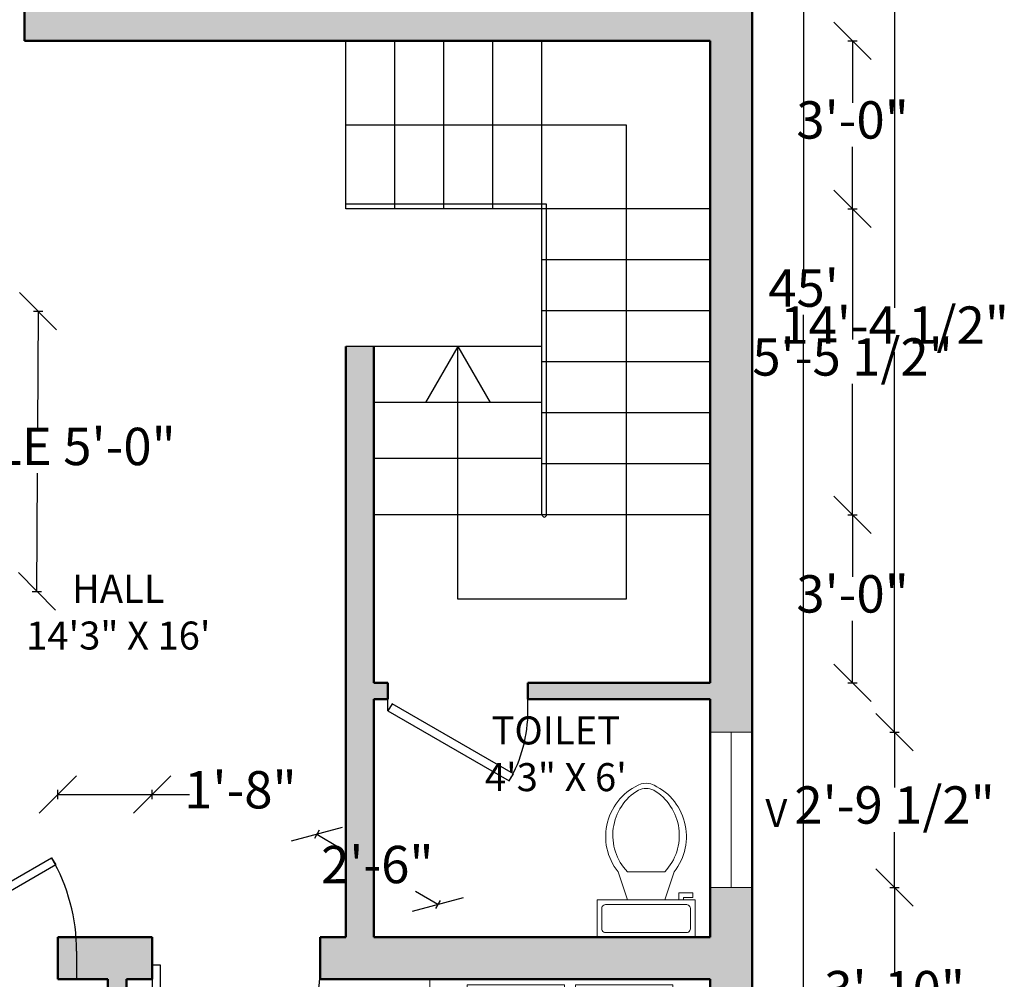
# Model space of a CAD drawing. Units: inches. Extents: x 3121 to 3511, y 1323 to 1998.
# Tile 8 of 10: x 3300 to 3511, y 1539 to 1744. Entities that reach past the tile are written whole.
import ezdxf

# ---------------------------------------------------------------- set-up
doc = ezdxf.new("R2010")
doc.units = ezdxf.units.IN
for name, color, linetype, lineweight in [('A-ANNO-DIMS', 2, 'Continuous', 18), ('A-ANNO-TEXT', 7, 'Continuous', 18), ('A-AREA-IDEN', 7, 'Continuous', 25), ('A-DOOR', 3, 'Continuous', 25), ('A-FLOR-FIXT', 9, 'Continuous', 18), ('A-FLOR-STRS', 7, 'Continuous', 25), ('A-FURN', 8, 'Continuous', 18), ('A-GLAZ', 4, 'Continuous', 18), ('A-WALL', 7, 'Continuous', 50), ('A-WALL-PATT', 3, 'Continuous', 13)]:
    doc.layers.add(name, color=color, linetype=linetype, lineweight=lineweight)
doc.styles.get("Standard").update_dxf_attribs({"font": 'arial.ttf'})
doc.dimstyles.new('ISO-25', dxfattribs={"dimtxt": 8, "dimasz": 8, "dimexe": 1, "dimexo": 1, "dimtad": 0, "dimtih": 1, "dimtoh": 1, "dimlunit": 3, "dimtxsty": 'Standard', "dimblk": 'OBLIQUE', "dimcen": 2.5, "dimclrt": 1, "dimadec": 0, "dimazin": 0, "dimtfac": 1, "dimtmove": 0, "dimatfit": 3, "dimfxl": 1, "dimfxlon": 1, "dimarcsym": 0})

# ---------------------------------------------------------------- blocks, each defined once
blk = doc.blocks.new('Bed - Queen')
for p, q in [((0, -80.00003), (0, 0)), ((0, 0), (59.99999, 0)), ((59.99999, 0), (59.99999, -80.00003)), ((7.99999, -1.2), (28.79998, -1.2)), ((7.99999, -14.4), (7.99999, -1.2)), ((28.79998, -1.2), (28.79998, -14.4)), ((31.19999, -1.2), (51.99999, -1.2)), ((31.19999, -14.4), (31.19999, -1.2)), ((51.99999, -1.2), (51.99999, -16.4)), ((0, -14.4), (44.8, -14.4)), ((59.99999, -29.6), (44.8, -14.4)), ((44.8, -14.4), (44.8, -29.6)), ((44.8, -16.8), (0, -16.8)), ((51.99999, -16.4), (46.79936, -16.4)), ((44.8, -29.6), (59.99999, -29.6)), ((59.99999, -80.00003), (0, -80.00003))]:
    blk.add_line(p, q)
blk = doc.blocks.new('Toilet - top')
for p, q in [((9.5, -6), (9.5, -2)), ((-8, -8.5), (-8, -8)), ((-7, -8), (-7, -9.5)), ((-4, -8), (-6, -14)), ((4, -8), (6, -14)), ((-10, -8.5), (-8, -8.5)), ((-10, -9.5), (-10, -8.5)), ((-7, -9.5), (-10, -9.5)), ((4, -14), (-4, -14))]:
    blk.add_line(p, q)
blk.add_lwpolyline([(10.5, -8), (10.5, 0), (-10.5, 0), (-10.5, -8)], close=True)
for points in [[(-9.5, -2), (-9.5, -6)], [(8.5, -1), (-8.5, -1)], [(-8.5, -7), (8.5, -7)]]:
    blk.add_lwpolyline(points)
for centre, radius, start, end in [((-8.62, -1.88), 0.884, 81.8699, 188.1301), ((8.62, -1.88), 0.884, 351.8699, 98.1301), ((-8.62, -6.12), 0.884, 171.8699, 278.1301), ((8.62, -6.12), 0.884, 261.8699, 8.1301), ((3.52, -21.58), 12.17, 141.4691, 247.9714), ((4.2, -21.82), 11.33, 136.3677, 238.9468), ((-3.52, -21.58), 12.17, 292.0284, 38.5307), ((-4.2, -21.82), 11.33, 301.053, 43.6321), ((0, -27.88), 4, 245.7318, 294.2682), ((0, -29), 4, 254.8605, 285.1395)]:
    blk.add_arc(centre, radius, start, end)
blk = doc.blocks.new('*U10')
for p, q in [((0, 0), (0, 6)), ((36, 0), (36, 6))]:
    blk.add_line(p, q)
blk.add_lwpolyline([(0, 0), (0, -36), (1.75, -36), (1.75, 0)], close=True)
blk.add_arc((0, 0), 36, 270, 0)
blk = doc.blocks.new('*U13')
for p, q in [((0, 0), (0, 6)), ((30, 0), (30, 6))]:
    blk.add_line(p, q)
blk.add_lwpolyline([(0, 0), (25.98, -15), (26.86, -13.48), (0.87, 1.52)], close=True)
blk.add_arc((0, 0), 30, 330, 0)
blk = doc.blocks.new('*U11')
for p, q in [((0, 0), (0, -6)), ((40, 0), (40, -6))]:
    blk.add_line(p, q)
blk.add_lwpolyline([(0, 0), (34.64, 20), (35.52, 18.48), (0.87, -1.52)], close=True)
blk.add_arc((0, 0), 40, 0, 30)
blk = doc.blocks.new('_Oblique')
at = {"color": 0, "linetype": 'ByBlock', "lineweight": -2}
blk.add_line((-0.5, -0.5), (0.5, 0.5), dxfattribs=at)
blk = doc.blocks.new('*D18')
at = {"layer": 'A-ANNO-DIMS', "color": 0, "lineweight": -2, "transparency": 16777216}
for p, q in [((3466.96, 1955.78), (3468.96, 1955.78)), ((3467.96, 1955.78), (3467.96, 1690.48)), ((3467.96, 1415.78), (3467.96, 1681.09)), ((3466.96, 1415.78), (3468.96, 1415.78))]:
    blk.add_line(p, q, dxfattribs=at)
at = {"layer": 'Defpoints', "color": 0, "transparency": 16777216}
for p in [(3456.92, 1955.78), (3456.92, 1415.78), (3467.96, 1415.78)]:
    blk.add_point(p, dxfattribs=at)
at = {"layer": 'A-ANNO-DIMS', "color": 0, "lineweight": -2, "transparency": 16777216, "xscale": 8, "yscale": 8, "zscale": 8}
for p, rotation in [((3467.96, 1955.78), 90), ((3467.96, 1415.78), 270)]:
    blk.add_blockref('_Oblique', p, dxfattribs=dict(at, rotation=rotation))
at = {"layer": 'A-ANNO-DIMS', "color": 0, "transparency": 16777216, "insert": (3467.96, 1685.78), "char_height": 8, "attachment_point": 5}
blk.add_mtext("45'", dxfattribs=at)
blk = doc.blocks.new('*D29')
at = {"layer": 'A-ANNO-DIMS', "color": 0, "lineweight": -2, "transparency": 16777216}
for p, q in [((3302.93, 1681.86), (3304.93, 1681.86)), ((3303.93, 1681.86), (3303.84, 1656.57)), ((3303.71, 1621.86), (3303.8, 1647.15)), ((3302.71, 1621.86), (3304.71, 1621.86))]:
    blk.add_line(p, q, dxfattribs=at)
at = {"layer": 'Defpoints', "color": 0, "transparency": 16777216}
for p in [(3294.93, 1681.89), (3303.93, 1681.86), (3294.71, 1621.89)]:
    blk.add_point(p, dxfattribs=at)
at = {"layer": 'A-ANNO-DIMS', "color": 0, "lineweight": -2, "transparency": 16777216, "xscale": 8, "yscale": 8, "zscale": 8}
for p, rotation in [((3303.93, 1681.86), 89.78583340711918), ((3303.71, 1621.86), 269.7858334071192)]:
    blk.add_blockref('_Oblique', p, dxfattribs=dict(at, rotation=rotation))
at = {"layer": 'A-ANNO-DIMS', "color": 1, "transparency": 16777216, "insert": (3303.82, 1651.86), "char_height": 8, "attachment_point": 5}
blk.add_mtext('TABLE 5\'-0"', dxfattribs=at)
blk = doc.blocks.new('*D46')
at = {"layer": 'A-ANNO-DIMS', "color": 0, "lineweight": -2, "transparency": 16777216}
for p, q in [((3486.47, 1558.43), (3488.47, 1558.43)), ((3487.47, 1558.43), (3487.47, 1540.24)), ((3487.47, 1512.63), (3487.47, 1530.82)), ((3486.47, 1512.63), (3488.47, 1512.63))]:
    blk.add_line(p, q, dxfattribs=at)
at = {"layer": 'Defpoints', "color": 0, "transparency": 16777216}
for p in [(3456.92, 1558.43), (3487.47, 1558.43), (3456.92, 1512.63)]:
    blk.add_point(p, dxfattribs=at)
at = {"layer": 'A-ANNO-DIMS', "color": 0, "lineweight": -2, "transparency": 16777216, "xscale": 8, "yscale": 8, "zscale": 8}
for p, rotation in [((3487.47, 1558.43), 90), ((3487.47, 1512.63), 270)]:
    blk.add_blockref('_Oblique', p, dxfattribs=dict(at, rotation=rotation))
at = {"layer": 'A-ANNO-DIMS', "color": 1, "transparency": 16777216, "insert": (3487.47, 1535.53), "char_height": 8, "attachment_point": 5}
blk.add_mtext('3\'-10"', dxfattribs=at)
blk = doc.blocks.new('*D47')
at = {"layer": 'A-ANNO-DIMS', "color": 0, "lineweight": -2, "transparency": 16777216}
for p, q in [((3486.47, 1591.7), (3488.47, 1591.7)), ((3487.47, 1591.7), (3487.47, 1579.83)), ((3487.47, 1558.43), (3487.47, 1570.3)), ((3486.47, 1558.43), (3488.47, 1558.43))]:
    blk.add_line(p, q, dxfattribs=at)
at = {"layer": 'Defpoints', "color": 0, "transparency": 16777216}
for p in [(3456.92, 1591.7), (3487.47, 1591.7), (3456.92, 1558.43)]:
    blk.add_point(p, dxfattribs=at)
at = {"layer": 'A-ANNO-DIMS', "color": 0, "lineweight": -2, "transparency": 16777216, "xscale": 8, "yscale": 8, "zscale": 8}
for p, rotation in [((3487.47, 1591.7), 90), ((3487.47, 1558.43), 270)]:
    blk.add_blockref('_Oblique', p, dxfattribs=dict(at, rotation=rotation))
at = {"layer": 'A-ANNO-DIMS', "color": 1, "transparency": 16777216, "insert": (3487.47, 1575.07), "char_height": 8, "attachment_point": 5}
blk.add_mtext('2\'-9 1/2"', dxfattribs=at)
blk = doc.blocks.new('*D48')
at = {"layer": 'A-ANNO-DIMS', "color": 0, "lineweight": -2, "transparency": 16777216}
for p, q in [((3486.47, 1763.99), (3488.47, 1763.99)), ((3487.47, 1763.99), (3487.47, 1682.6)), ((3487.47, 1591.7), (3487.47, 1673.08)), ((3486.47, 1591.7), (3488.47, 1591.7))]:
    blk.add_line(p, q, dxfattribs=at)
at = {"layer": 'Defpoints', "color": 0, "transparency": 16777216}
for p in [(3456.92, 1763.99), (3487.47, 1763.99), (3456.92, 1591.7)]:
    blk.add_point(p, dxfattribs=at)
at = {"layer": 'A-ANNO-DIMS', "color": 0, "lineweight": -2, "transparency": 16777216, "xscale": 8, "yscale": 8, "zscale": 8}
for p, rotation in [((3487.47, 1763.99), 90), ((3487.47, 1591.7), 270)]:
    blk.add_blockref('_Oblique', p, dxfattribs=dict(at, rotation=rotation))
at = {"layer": 'A-ANNO-DIMS', "color": 1, "transparency": 16777216, "insert": (3487.47, 1677.84), "char_height": 8, "attachment_point": 5}
blk.add_mtext('14\'-4 1/2"', dxfattribs=at)
blk = doc.blocks.new('*D53')
at = {"layer": 'A-ANNO-DIMS', "color": 0, "lineweight": -2, "transparency": 16777216}
for p, q in [((3274.02, 1336.37), (3274.02, 1334.37)), ((3310.02, 1336.37), (3310.02, 1334.37)), ((3274.02, 1335.37), (3280.77, 1335.37)), ((3310.02, 1335.37), (3303.28, 1335.37))]:
    blk.add_line(p, q, dxfattribs=at)
at = {"layer": 'Defpoints', "color": 0, "transparency": 16777216}
for p in [(3274.02, 1946.78), (3310.02, 1946.78), (3310.02, 1335.37)]:
    blk.add_point(p, dxfattribs=at)
at = {"layer": 'A-ANNO-DIMS', "color": 0, "lineweight": -2, "transparency": 16777216, "xscale": 8, "yscale": 8, "zscale": 8, "rotation": 180}
blk.add_blockref('_Oblique', (3274.02, 1335.37), dxfattribs=at)
at = {"layer": 'A-ANNO-DIMS', "color": 0, "lineweight": -2, "transparency": 16777216, "xscale": 8, "yscale": 8, "zscale": 8}
blk.add_blockref('_Oblique', (3310.02, 1335.37), dxfattribs=at)
at = {"layer": 'A-ANNO-DIMS', "color": 1, "transparency": 16777216, "insert": (3292.02, 1335.37), "char_height": 8, "attachment_point": 5}
blk.add_mtext('3\'-0"', dxfattribs=at)
blk = doc.blocks.new('*D54')
at = {"layer": 'A-ANNO-DIMS', "color": 0, "lineweight": -2, "transparency": 16777216}
for p, q in [((3310.02, 1336.37), (3310.02, 1334.37)), ((3334.16, 1336.37), (3334.16, 1334.37)), ((3310.02, 1335.37), (3310.76, 1335.37)), ((3334.16, 1335.37), (3333.42, 1335.37))]:
    blk.add_line(p, q, dxfattribs=at)
at = {"layer": 'Defpoints', "color": 0, "transparency": 16777216}
for p in [(3310.02, 1946.78), (3334.16, 1946.78), (3334.16, 1335.37)]:
    blk.add_point(p, dxfattribs=at)
at = {"layer": 'A-ANNO-DIMS', "color": 0, "lineweight": -2, "transparency": 16777216, "xscale": 8, "yscale": 8, "zscale": 8, "rotation": 180}
blk.add_blockref('_Oblique', (3310.02, 1335.37), dxfattribs=at)
at = {"layer": 'A-ANNO-DIMS', "color": 0, "lineweight": -2, "transparency": 16777216, "xscale": 8, "yscale": 8, "zscale": 8}
blk.add_blockref('_Oblique', (3334.16, 1335.37), dxfattribs=at)
at = {"layer": 'A-ANNO-DIMS', "color": 1, "transparency": 16777216, "insert": (3322.09, 1335.37), "char_height": 8, "attachment_point": 5}
blk.add_mtext('2\'-0"', dxfattribs=at)
blk = doc.blocks.new('*D55')
at = {"layer": 'A-ANNO-DIMS', "color": 0, "lineweight": -2, "transparency": 16777216}
for p, q in [((3334.16, 1336.37), (3334.16, 1334.37)), ((3384.56, 1336.37), (3384.56, 1334.37)), ((3334.16, 1335.37), (3338.62, 1335.37)), ((3384.56, 1335.37), (3380.1, 1335.37))]:
    blk.add_line(p, q, dxfattribs=at)
at = {"layer": 'Defpoints', "color": 0, "transparency": 16777216}
for p in [(3334.16, 1946.78), (3384.56, 1946.78), (3384.56, 1335.37)]:
    blk.add_point(p, dxfattribs=at)
at = {"layer": 'A-ANNO-DIMS', "color": 0, "lineweight": -2, "transparency": 16777216, "xscale": 8, "yscale": 8, "zscale": 8, "rotation": 180}
blk.add_blockref('_Oblique', (3334.16, 1335.37), dxfattribs=at)
at = {"layer": 'A-ANNO-DIMS', "color": 0, "lineweight": -2, "transparency": 16777216, "xscale": 8, "yscale": 8, "zscale": 8}
blk.add_blockref('_Oblique', (3384.56, 1335.37), dxfattribs=at)
at = {"layer": 'A-ANNO-DIMS', "color": 1, "transparency": 16777216, "insert": (3359.36, 1335.37), "char_height": 8, "attachment_point": 5}
blk.add_mtext('4\'-2 1/2"', dxfattribs=at)
blk = doc.blocks.new('*D58')
at = {"layer": 'A-ANNO-DIMS', "color": 0, "lineweight": -2, "transparency": 16777216}
for p, q in [((3209.89, 1985.33), (3209.89, 1987.33)), ((3209.89, 1986.33), (3240.03, 1986.33)), ((3311.33, 1986.33), (3281.19, 1986.33)), ((3311.33, 1985.33), (3311.33, 1987.33))]:
    blk.add_line(p, q, dxfattribs=at)
at = {"layer": 'Defpoints', "color": 0, "transparency": 16777216}
for p in [(3311.33, 1986.33), (3209.89, 1424.78), (3311.33, 1424.78)]:
    blk.add_point(p, dxfattribs=at)
at = {"layer": 'A-ANNO-DIMS', "color": 0, "lineweight": -2, "transparency": 16777216, "xscale": 8, "yscale": 8, "zscale": 8, "rotation": 180}
blk.add_blockref('_Oblique', (3209.89, 1986.33), dxfattribs=at)
at = {"layer": 'A-ANNO-DIMS', "color": 0, "lineweight": -2, "transparency": 16777216, "xscale": 8, "yscale": 8, "zscale": 8}
blk.add_blockref('_Oblique', (3311.33, 1986.33), dxfattribs=at)
at = {"layer": 'A-ANNO-DIMS', "color": 1, "transparency": 16777216, "insert": (3260.61, 1986.33), "char_height": 8, "attachment_point": 5}
blk.add_mtext('8\'-5 1/2"', dxfattribs=at)
blk = doc.blocks.new('*D59')
at = {"layer": 'A-ANNO-DIMS', "color": 0, "lineweight": -2, "transparency": 16777216}
for p, q in [((3318.92, 1336.37), (3318.92, 1334.37)), ((3370.92, 1336.37), (3370.92, 1334.37)), ((3318.92, 1335.37), (3333.5, 1335.37)), ((3370.92, 1335.37), (3356.34, 1335.37))]:
    blk.add_line(p, q, dxfattribs=at)
at = {"layer": 'Defpoints', "color": 0, "transparency": 16777216}
for p in [(3318.92, 1752.23), (3370.92, 1748.78), (3370.92, 1335.37)]:
    blk.add_point(p, dxfattribs=at)
at = {"layer": 'A-ANNO-DIMS', "color": 0, "lineweight": -2, "transparency": 16777216, "xscale": 8, "yscale": 8, "zscale": 8, "rotation": 180}
blk.add_blockref('_Oblique', (3318.92, 1335.37), dxfattribs=at)
at = {"layer": 'A-ANNO-DIMS', "color": 0, "lineweight": -2, "transparency": 16777216, "xscale": 8, "yscale": 8, "zscale": 8}
blk.add_blockref('_Oblique', (3370.92, 1335.37), dxfattribs=at)
at = {"layer": 'A-ANNO-DIMS', "color": 1, "transparency": 16777216, "insert": (3344.92, 1335.37), "char_height": 8, "attachment_point": 5}
blk.add_mtext('4\'-4"', dxfattribs=at)
blk = doc.blocks.new('*D63')
at = {"layer": 'A-ANNO-DIMS', "color": 0, "lineweight": -2, "transparency": 16777216}
for p, q in [((3370.92, 1336.37), (3370.92, 1334.37)), ((3379.92, 1336.37), (3379.92, 1334.37)), ((3370.92, 1335.37), (3379.92, 1335.37)), ((3379.92, 1335.37), (3387.92, 1335.37))]:
    blk.add_line(p, q, dxfattribs=at)
at = {"layer": 'Defpoints', "color": 0, "transparency": 16777216}
for p in [(3370.92, 1748.78), (3379.92, 1748.78), (3379.92, 1335.37)]:
    blk.add_point(p, dxfattribs=at)
at = {"layer": 'A-ANNO-DIMS', "color": 0, "lineweight": -2, "transparency": 16777216, "xscale": 8, "yscale": 8, "zscale": 8, "rotation": 180}
blk.add_blockref('_Oblique', (3370.92, 1335.37), dxfattribs=at)
at = {"layer": 'A-ANNO-DIMS', "color": 0, "lineweight": -2, "transparency": 16777216, "xscale": 8, "yscale": 8, "zscale": 8}
blk.add_blockref('_Oblique', (3379.92, 1335.37), dxfattribs=at)
at = {"layer": 'A-ANNO-DIMS', "color": 1, "transparency": 16777216, "insert": (3399.18, 1335.37), "char_height": 8, "attachment_point": 5}
blk.add_mtext('0\'-9"', dxfattribs=at)
blk = doc.blocks.new('*D64')
at = {"layer": 'A-ANNO-DIMS', "color": 0, "lineweight": -2, "transparency": 16777216}
for p, q in [((3411.92, 1336.37), (3411.92, 1334.37)), ((3447.92, 1336.37), (3447.92, 1334.37)), ((3411.92, 1335.37), (3418.66, 1335.37)), ((3447.92, 1335.37), (3441.17, 1335.37))]:
    blk.add_line(p, q, dxfattribs=at)
at = {"layer": 'Defpoints', "color": 0, "transparency": 16777216}
for p in [(3411.92, 1638.28), (3447.92, 1638.28), (3447.92, 1335.37)]:
    blk.add_point(p, dxfattribs=at)
at = {"layer": 'A-ANNO-DIMS', "color": 0, "lineweight": -2, "transparency": 16777216, "xscale": 8, "yscale": 8, "zscale": 8, "rotation": 180}
blk.add_blockref('_Oblique', (3411.92, 1335.37), dxfattribs=at)
at = {"layer": 'A-ANNO-DIMS', "color": 0, "lineweight": -2, "transparency": 16777216, "xscale": 8, "yscale": 8, "zscale": 8}
blk.add_blockref('_Oblique', (3447.92, 1335.37), dxfattribs=at)
at = {"layer": 'A-ANNO-DIMS', "color": 1, "transparency": 16777216, "insert": (3429.92, 1335.37), "char_height": 8, "attachment_point": 5}
blk.add_mtext('3\'-0"', dxfattribs=at)
blk = doc.blocks.new('*D65')
at = {"layer": 'A-ANNO-DIMS', "color": 0, "lineweight": -2, "transparency": 16777216}
for p, q in [((3477.47, 1739.78), (3479.47, 1739.78)), ((3478.47, 1739.78), (3478.47, 1726.5)), ((3478.47, 1703.78), (3478.47, 1717.07)), ((3477.47, 1703.78), (3479.47, 1703.78))]:
    blk.add_line(p, q, dxfattribs=at)
at = {"layer": 'Defpoints', "color": 0, "transparency": 16777216}
for p in [(3447.92, 1739.78), (3447.92, 1703.78), (3478.47, 1703.78)]:
    blk.add_point(p, dxfattribs=at)
at = {"layer": 'A-ANNO-DIMS', "color": 0, "lineweight": -2, "transparency": 16777216, "xscale": 8, "yscale": 8, "zscale": 8}
for p, rotation in [((3478.47, 1739.78), 90), ((3478.47, 1703.78), 270)]:
    blk.add_blockref('_Oblique', p, dxfattribs=dict(at, rotation=rotation))
at = {"layer": 'A-ANNO-DIMS', "color": 1, "transparency": 16777216, "insert": (3478.47, 1721.78), "char_height": 8, "attachment_point": 5}
blk.add_mtext('3\'-0"', dxfattribs=at)
blk = doc.blocks.new('*D66')
at = {"layer": 'A-ANNO-DIMS', "color": 0, "lineweight": -2, "transparency": 16777216}
for p, q in [((3477.47, 1638.28), (3479.47, 1638.28)), ((3478.47, 1638.28), (3478.47, 1625)), ((3478.47, 1602.28), (3478.47, 1615.57)), ((3477.47, 1602.28), (3479.47, 1602.28))]:
    blk.add_line(p, q, dxfattribs=at)
at = {"layer": 'Defpoints', "color": 0, "transparency": 16777216}
for p in [(3447.92, 1638.28), (3447.92, 1602.28), (3478.47, 1602.28)]:
    blk.add_point(p, dxfattribs=at)
at = {"layer": 'A-ANNO-DIMS', "color": 0, "lineweight": -2, "transparency": 16777216, "xscale": 8, "yscale": 8, "zscale": 8}
for p, rotation in [((3478.47, 1638.28), 90), ((3478.47, 1602.28), 270)]:
    blk.add_blockref('_Oblique', p, dxfattribs=dict(at, rotation=rotation))
at = {"layer": 'A-ANNO-DIMS', "color": 1, "transparency": 16777216, "insert": (3478.47, 1620.28), "char_height": 8, "attachment_point": 5}
blk.add_mtext('3\'-0"', dxfattribs=at)
blk = doc.blocks.new('*D71')
at = {"layer": 'A-ANNO-DIMS', "color": 0, "lineweight": -2, "transparency": 16777216}
for p, q in [((3308.21, 1577.33), (3308.21, 1579.33)), ((3308.21, 1578.33), (3328.42, 1578.33)), ((3328.42, 1577.33), (3328.42, 1579.33)), ((3328.42, 1578.33), (3336.42, 1578.33))]:
    blk.add_line(p, q, dxfattribs=at)
at = {"layer": 'Defpoints', "color": 0, "transparency": 16777216}
for p in [(3328.42, 1578.33), (3308.21, 1547.78), (3328.42, 1547.78)]:
    blk.add_point(p, dxfattribs=at)
at = {"layer": 'A-ANNO-DIMS', "color": 0, "lineweight": -2, "transparency": 16777216, "xscale": 8, "yscale": 8, "zscale": 8, "rotation": 180}
blk.add_blockref('_Oblique', (3308.21, 1578.33), dxfattribs=at)
at = {"layer": 'A-ANNO-DIMS', "color": 0, "lineweight": -2, "transparency": 16777216, "xscale": 8, "yscale": 8, "zscale": 8}
blk.add_blockref('_Oblique', (3328.42, 1578.33), dxfattribs=at)
at = {"layer": 'A-ANNO-DIMS', "color": 1, "transparency": 16777216, "insert": (3347.3, 1578.33), "char_height": 8, "attachment_point": 5}
blk.add_mtext('1\'-8"', dxfattribs=at)
blk = doc.blocks.new('*D73')
at = {"layer": 'A-ANNO-DIMS', "color": 0, "lineweight": -2, "transparency": 16777216}
for p, q in [((3261.02, 1336.37), (3261.02, 1334.37)), ((3301.03, 1336.37), (3301.03, 1334.37)), ((3261.02, 1335.37), (3269.77, 1335.37)), ((3301.03, 1335.37), (3292.28, 1335.37))]:
    blk.add_line(p, q, dxfattribs=at)
at = {"layer": 'Defpoints', "color": 0, "transparency": 16777216}
for p in [(3261.02, 1739.78), (3301.03, 1739.78), (3301.03, 1335.37)]:
    blk.add_point(p, dxfattribs=at)
at = {"layer": 'A-ANNO-DIMS', "color": 0, "lineweight": -2, "transparency": 16777216, "xscale": 8, "yscale": 8, "zscale": 8, "rotation": 180}
blk.add_blockref('_Oblique', (3261.02, 1335.37), dxfattribs=at)
at = {"layer": 'A-ANNO-DIMS', "color": 0, "lineweight": -2, "transparency": 16777216, "xscale": 8, "yscale": 8, "zscale": 8}
blk.add_blockref('_Oblique', (3301.03, 1335.37), dxfattribs=at)
at = {"layer": 'A-ANNO-DIMS', "color": 1, "transparency": 16777216, "insert": (3281.02, 1335.37), "char_height": 8, "attachment_point": 5}
blk.add_mtext('3\'-4"', dxfattribs=at)
blk = doc.blocks.new('*D74')
at = {"layer": 'A-ANNO-DIMS', "color": 0, "lineweight": -2, "transparency": 16777216}
for p, q in [((3375.92, 1985.33), (3375.92, 1987.33)), ((3375.92, 1986.33), (3382.66, 1986.33)), ((3411.92, 1986.33), (3405.17, 1986.33)), ((3411.92, 1985.33), (3411.92, 1987.33))]:
    blk.add_line(p, q, dxfattribs=at)
at = {"layer": 'Defpoints', "color": 0, "transparency": 16777216}
for p in [(3411.92, 1986.33), (3375.92, 1674.28), (3411.92, 1674.28)]:
    blk.add_point(p, dxfattribs=at)
at = {"layer": 'A-ANNO-DIMS', "color": 0, "lineweight": -2, "transparency": 16777216, "xscale": 8, "yscale": 8, "zscale": 8, "rotation": 180}
blk.add_blockref('_Oblique', (3375.92, 1986.33), dxfattribs=at)
at = {"layer": 'A-ANNO-DIMS', "color": 0, "lineweight": -2, "transparency": 16777216, "xscale": 8, "yscale": 8, "zscale": 8}
blk.add_blockref('_Oblique', (3411.92, 1986.33), dxfattribs=at)
at = {"layer": 'A-ANNO-DIMS', "color": 1, "transparency": 16777216, "insert": (3393.92, 1986.33), "char_height": 8, "attachment_point": 5}
blk.add_mtext('3\'-0"', dxfattribs=at)
blk = doc.blocks.new('*D75')
at = {"layer": 'A-ANNO-DIMS', "color": 0, "lineweight": -2, "transparency": 16777216}
for p, q in [((3369.92, 1336.37), (3369.92, 1334.37)), ((3411.92, 1336.37), (3411.92, 1334.37)), ((3369.92, 1335.37), (3379.66, 1335.37)), ((3411.92, 1335.37), (3402.17, 1335.37))]:
    blk.add_line(p, q, dxfattribs=at)
at = {"layer": 'Defpoints', "color": 0, "transparency": 16777216}
for p in [(3369.92, 1703.78), (3411.92, 1703.78), (3411.92, 1335.37)]:
    blk.add_point(p, dxfattribs=at)
at = {"layer": 'A-ANNO-DIMS', "color": 0, "lineweight": -2, "transparency": 16777216, "xscale": 8, "yscale": 8, "zscale": 8, "rotation": 180}
blk.add_blockref('_Oblique', (3369.92, 1335.37), dxfattribs=at)
at = {"layer": 'A-ANNO-DIMS', "color": 0, "lineweight": -2, "transparency": 16777216, "xscale": 8, "yscale": 8, "zscale": 8}
blk.add_blockref('_Oblique', (3411.92, 1335.37), dxfattribs=at)
at = {"layer": 'A-ANNO-DIMS', "color": 1, "transparency": 16777216, "insert": (3390.92, 1335.37), "char_height": 8, "attachment_point": 5}
blk.add_mtext('3\'-6"', dxfattribs=at)
blk = doc.blocks.new('*D76')
at = {"layer": 'A-ANNO-DIMS', "color": 0, "lineweight": -2, "transparency": 16777216}
for p, q in [((3477.47, 1703.78), (3479.47, 1703.78)), ((3478.47, 1703.78), (3478.47, 1675.8)), ((3478.47, 1638.28), (3478.47, 1666.27)), ((3477.47, 1638.28), (3479.47, 1638.28))]:
    blk.add_line(p, q, dxfattribs=at)
at = {"layer": 'Defpoints', "color": 0, "transparency": 16777216}
for p in [(3447.92, 1703.78), (3447.92, 1638.28), (3478.47, 1638.28)]:
    blk.add_point(p, dxfattribs=at)
at = {"layer": 'A-ANNO-DIMS', "color": 0, "lineweight": -2, "transparency": 16777216, "xscale": 8, "yscale": 8, "zscale": 8}
for p, rotation in [((3478.47, 1703.78), 90), ((3478.47, 1638.28), 270)]:
    blk.add_blockref('_Oblique', p, dxfattribs=dict(at, rotation=rotation))
at = {"layer": 'A-ANNO-DIMS', "color": 1, "transparency": 16777216, "insert": (3478.47, 1671.03), "char_height": 8, "attachment_point": 5}
blk.add_mtext('5\'-5 1/2"', dxfattribs=at)
blk = doc.blocks.new('*D77')
at = {"layer": 'A-ANNO-DIMS', "color": 0, "lineweight": -2, "transparency": 16777216}
for p, q in [((3364.14, 1570.69), (3363.14, 1568.96)), ((3363.64, 1569.83), (3368.48, 1567.04)), ((3389.62, 1554.83), (3384.79, 1557.62)), ((3390.12, 1555.69), (3389.12, 1553.96))]:
    blk.add_line(p, q, dxfattribs=at)
at = {"layer": 'Defpoints', "color": 0, "transparency": 16777216}
for p in [(3378.92, 1596.28), (3404.9, 1581.28), (3363.64, 1569.83)]:
    blk.add_point(p, dxfattribs=at)
at = {"layer": 'A-ANNO-DIMS', "color": 0, "lineweight": -2, "transparency": 16777216, "xscale": 8, "yscale": 8, "zscale": 8}
for p, rotation in [((3363.64, 1569.83), 150.0000000000001), ((3389.62, 1554.83), 330.0000000000001)]:
    blk.add_blockref('_Oblique', p, dxfattribs=dict(at, rotation=rotation))
at = {"layer": 'A-ANNO-DIMS', "color": 1, "transparency": 16777216, "insert": (3376.63, 1562.33), "char_height": 8, "attachment_point": 5}
blk.add_mtext('2\'-6"', dxfattribs=at)

msp = doc.modelspace()

# ---------------------------------------------------------------- hatches: boundary and pattern name
at = {"layer": 'A-WALL-PATT'}
h = msp.add_hatch(color=256, dxfattribs=at)
h.dxf.hatch_style = 1
h.paths.add_polyline_path([(3274.023, 1955.784), (3189.918, 1955.784), (3189.918, 1910.219), (3198.918, 1910.219), (3198.918, 1946.784), (3259.023, 1946.784), (3259.023, 1921.61), (3261.023, 1921.61), (3261.023, 1946.784), (3274.023, 1946.784)])
h.paths.add_polyline_path([(3327.918, 1946.784), (3334.156, 1946.784), (3334.156, 1955.784), (3310.023, 1955.784), (3310.023, 1946.784), (3318.918, 1946.784), (3318.918, 1929.796), (3311.644, 1929.796), (3311.644, 1927.007), (3324.033, 1927.007), (3324.033, 1871.381), (3311.644, 1871.381), (3311.644, 1868.381), (3318.918, 1868.381), (3318.918, 1853.784), (3327.918, 1853.784)])
h.paths.add_polyline_path([(3456.918, 1955.784), (3384.562, 1955.784), (3384.562, 1946.784), (3447.918, 1946.784), (3447.918, 1877.779), (3456.918, 1877.779)])
h.paths.add_polyline_path([(3456.918, 1835.782), (3447.918, 1835.782), (3447.918, 1814.784), (3414.918, 1814.784), (3414.918, 1803.784), (3447.918, 1803.784), (3447.918, 1793.443), (3456.918, 1793.443)])
h.paths.add_polyline_path([(3456.918, 1558.434), (3447.918, 1558.434), (3447.918, 1547.784), (3375.918, 1547.784), (3375.918, 1598.784), (3378.918, 1598.784), (3378.918, 1602.284), (3375.918, 1602.284), (3375.918, 1674.284), (3369.918, 1674.284), (3369.918, 1547.784), (3364.418, 1547.784), (3364.418, 1538.784), (3447.918, 1538.784), (3447.918, 1512.628), (3456.918, 1512.628)])
h.paths.add_polyline_path([(3456.918, 1460.558), (3447.918, 1460.558), (3447.918, 1424.784), (3412.543, 1424.784), (3412.543, 1415.784), (3456.918, 1415.784)])
h.paths.add_polyline_path([(3358.149, 1424.784), (3322.918, 1424.784), (3322.918, 1538.784), (3328.418, 1538.784), (3328.418, 1547.784), (3308.208, 1547.784), (3308.208, 1538.784), (3318.918, 1538.784), (3318.918, 1424.784), (3311.328, 1424.784), (3311.328, 1415.784), (3358.149, 1415.784)])
h.paths.add_polyline_path([(3207.562, 1547.784), (3198.918, 1547.784), (3198.918, 1607.327), (3189.918, 1607.327), (3189.918, 1513.073), (3198.918, 1513.073), (3198.918, 1538.784), (3207.562, 1538.784)])
h.paths.add_polyline_path([(3198.918, 1461.548), (3189.918, 1461.548), (3189.918, 1415.784), (3209.892, 1415.784), (3209.892, 1424.784), (3198.918, 1424.784)])
h.paths.add_polyline_path([(3272.208, 1547.784), (3238.766, 1547.784), (3238.766, 1538.784), (3272.208, 1538.784)])
h.paths.add_polyline_path([(3261.023, 1748.784), (3198.918, 1748.784), (3198.918, 1768.387), (3189.918, 1768.387), (3189.918, 1692.279), (3198.918, 1692.279), (3198.918, 1739.784), (3261.023, 1739.784)])
h.paths.add_polyline_path([(3198.918, 1856.171), (3189.918, 1856.171), (3189.918, 1808.331), (3198.918, 1808.331), (3198.918, 1821.074), (3261.023, 1821.074), (3261.023, 1862.309), (3259.023, 1862.309), (3259.023, 1825.074), (3198.918, 1825.074)])
h = msp.add_hatch(color=256, dxfattribs=at)
h.dxf.hatch_style = 1
h.paths.add_polyline_path([(3382.918, 1814.784), (3327.918, 1814.784), (3327.918, 1817.784), (3318.918, 1817.784), (3318.918, 1800.224), (3324.918, 1800.224), (3327.918, 1800.224), (3327.918, 1803.784), (3370.918, 1803.784), (3370.918, 1748.784), (3327.918, 1748.784), (3327.918, 1752.226), (3324.918, 1752.226), (3318.918, 1752.226), (3318.918, 1748.784), (3301.026, 1748.784), (3301.026, 1739.784), (3447.918, 1739.784), (3447.918, 1602.284), (3418.918, 1602.284), (3418.918, 1598.784), (3447.918, 1598.784), (3447.918, 1591.697), (3456.918, 1591.697), (3456.918, 1763.985), (3447.918, 1763.985), (3447.918, 1748.784), (3379.918, 1748.784), (3379.918, 1803.784), (3382.918, 1803.784)])
h.paths.add_polyline_path([(3418.918, 1602.284), (3408.918, 1602.284), (3408.918, 1598.784), (3418.918, 1598.784)], flags=17)

# ---------------------------------------------------------------- linework, layer by layer
at = {"layer": 'A-FLOR-STRS'}
for p, q in [((3369.918, 1703.784), (3369.918, 1739.784)), ((3380.418, 1703.784), (3380.418, 1739.784)), ((3390.918, 1703.784), (3390.918, 1739.784)), ((3401.418, 1703.784), (3401.418, 1739.784)), ((3411.918, 1703.784), (3411.918, 1739.784)), ((3369.918, 1721.784), (3429.918, 1721.784)), ((3429.918, 1721.784), (3429.918, 1620.186)), ((3412.918, 1704.784), (3369.918, 1704.784)), ((3412.918, 1638.284), (3412.918, 1704.784)), ((3411.918, 1703.784), (3369.918, 1703.784)), ((3447.918, 1703.784), (3411.918, 1703.784)), ((3411.918, 1638.284), (3411.918, 1703.784)), ((3447.918, 1692.867), (3411.918, 1692.867)), ((3447.918, 1681.951), (3411.918, 1681.951)), ((3411.918, 1674.284), (3369.918, 1674.284)), ((3393.918, 1674.284), (3386.99, 1662.284)), ((3393.918, 1620.186), (3393.918, 1674.284)), ((3393.918, 1674.284), (3400.846, 1662.284)), ((3447.918, 1671.034), (3411.918, 1671.034)), ((3411.918, 1662.284), (3375.918, 1662.284)), ((3447.918, 1660.117), (3411.918, 1660.117)), ((3411.918, 1650.284), (3375.918, 1650.284)), ((3447.918, 1649.201), (3411.918, 1649.201)), ((3447.918, 1638.284), (3375.918, 1638.284)), ((3411.918, 1638.284), (3375.918, 1638.284)), ((3429.918, 1620.186), (3393.918, 1620.186))]:
    msp.add_line(p, q, dxfattribs=at)
msp.add_arc((3412.418, 1638.284), 0.5, 180, 0, dxfattribs=at)
at = {"layer": 'A-GLAZ'}
for p, q in [((3447.918, 1591.697), (3456.918, 1591.697)), ((3452.418, 1558.434), (3452.418, 1591.697)), ((3447.918, 1558.434), (3456.918, 1558.434))]:
    msp.add_line(p, q, dxfattribs=at)
at = {"layer": 'A-WALL'}
for p, q in [((3456.918, 1415.784), (3456.918, 1955.784)), ((3301.026, 1748.784), (3301.026, 1739.784)), ((3447.918, 1739.784), (3301.026, 1739.784)), ((3447.918, 1602.284), (3447.918, 1739.784)), ((3369.918, 1674.284), (3369.918, 1547.784)), ((3375.918, 1674.284), (3375.918, 1602.284)), ((3378.918, 1602.284), (3375.918, 1602.284)), ((3378.918, 1602.284), (3378.918, 1598.784)), ((3447.918, 1602.284), (3408.918, 1602.284)), ((3408.918, 1602.284), (3408.918, 1598.784)), ((3375.918, 1598.784), (3375.918, 1547.784)), ((3378.918, 1598.784), (3375.918, 1598.784)), ((3447.918, 1598.784), (3408.918, 1598.784)), ((3447.918, 1547.784), (3447.918, 1598.784)), ((3308.208, 1538.784), (3308.208, 1547.784)), ((3328.418, 1547.784), (3308.208, 1547.784)), ((3328.418, 1538.784), (3328.418, 1547.784)), ((3369.918, 1547.784), (3364.418, 1547.784)), ((3364.418, 1538.784), (3364.418, 1547.784)), ((3447.918, 1547.784), (3375.918, 1547.784)), ((3318.918, 1538.784), (3308.208, 1538.784)), ((3318.918, 1424.784), (3318.918, 1538.784)), ((3322.918, 1424.784), (3322.918, 1538.784)), ((3328.418, 1538.784), (3322.918, 1538.784)), ((3447.918, 1538.784), (3364.418, 1538.784)), ((3447.918, 1424.784), (3447.918, 1538.784))]:
    msp.add_line(p, q, dxfattribs=at)

# ---------------------------------------------------------------- block references
at = {"layer": 'A-DOOR'}
for name, p in [('*U13', (3378.918, 1596.284)), ('*U11', (3272.208, 1544.784)), ('*U10', (3328.418, 1541.784))]:
    msp.add_blockref(name, p, dxfattribs=at)
at = {"layer": 'A-FLOR-FIXT', "rotation": 180}
msp.add_blockref('Toilet - top', (3434.216, 1547.784), dxfattribs=at)
at = {"layer": 'A-FURN'}
msp.add_blockref('Bed - Queen', (3387.918, 1538.784), dxfattribs=at)

# ---------------------------------------------------------------- texts
at = {"layer": 'A-ANNO-TEXT', "insert": (3455.916, 1577.402), "char_height": 6, "attachment_point": 1}
msp.add_mtext_dynamic_manual_height_columns('\\pxqc;V', width=12.42925, gutter_width=12.5, heights=[0], dxfattribs=at)
at = {"layer": 'A-AREA-IDEN', "char_height": 6, "attachment_point": 1}
for s, insert in [('\\pxqc;HALL\\P14\'3" X 16\'', (3286.317, 1625.402)), ('\\pxqc;TOILET\\P4\'3" X 6\'', (3380.063, 1595.077))]:
    msp.add_mtext_dynamic_manual_height_columns(s, width=69.63762, gutter_width=12.5, heights=[0], dxfattribs=dict(at, insert=insert))

# ---------------------------------------------------------------- dimensions: what is measured, and where the dimension line sits
at = {"layer": 'A-ANNO-DIMS'}
for base, p1, p2, picture, middle in [((3311.328, 1986.334), (3209.892, 1424.784), (3311.328, 1424.784), '*D58', (3260.61, 1986.334)), ((3411.918, 1986.334), (3375.918, 1674.284), (3411.918, 1674.284), '*D74', (3393.918, 1986.334)), ((3310.023, 1335.367), (3274.023, 1946.784), (3310.023, 1946.784), '*D53', (3292.023, 1335.367)), ((3334.156, 1335.367), (3310.023, 1946.784), (3334.156, 1946.784), '*D54', (3322.089, 1335.367)), ((3384.562, 1335.367), (3334.156, 1946.784), (3384.562, 1946.784), '*D55', (3359.359, 1335.367)), ((3370.918, 1335.367), (3318.918, 1752.226), (3370.918, 1748.784), '*D59', (3344.918, 1335.367)), ((3379.918, 1335.367), (3370.918, 1748.784), (3379.918, 1748.784), '*D63', (3399.176, 1335.367)), ((3301.026, 1335.367), (3261.023, 1739.784), (3301.026, 1739.784), '*D73', (3281.024, 1335.367)), ((3411.918, 1335.367), (3369.918, 1703.784), (3411.918, 1703.784), '*D75', (3390.918, 1335.367)), ((3447.918, 1335.367), (3411.918, 1638.284), (3447.918, 1638.284), '*D64', (3429.918, 1335.367)), ((3328.418, 1578.334), (3308.208, 1547.784), (3328.418, 1547.784), '*D71', (3347.299, 1578.334))]:
    dim = msp.add_linear_dim(base=base, p1=p1, p2=p2, dimstyle='ISO-25', override={"dimdec": 1, "dimlfac": 1, "dimrnd": 0, "dimzin": 1, "dimdsep": 46, "dimlunit": 4, "dimfrac": 2}, dxfattribs=at)
    dim.commit()
    dim.dimension.update_dxf_attribs({"geometry": picture, "text_midpoint": middle})
for base, p1, p2, angle, override, picture, middle in [((3467.957, 1415.784), (3456.918, 1955.784), (3456.918, 1415.784), 90, {"dimclrd": 0, "dimclre": 0, "dimclrt": 0}, '*D18', (3467.957, 1685.784)), ((3487.468, 1763.985), (3456.918, 1591.697), (3456.918, 1763.985), 90, {"dimdec": 1, "dimlfac": 1, "dimrnd": 0, "dimzin": 1, "dimdsep": 46, "dimlunit": 4, "dimfrac": 2}, '*D48', (3487.468, 1677.841)), ((3478.468, 1703.784), (3447.918, 1739.784), (3447.918, 1703.784), 270, {"dimdec": 1, "dimlfac": 1, "dimrnd": 0, "dimzin": 1, "dimdsep": 46, "dimlunit": 4, "dimfrac": 2}, '*D65', (3478.468, 1721.784)), ((3478.468, 1638.284), (3447.918, 1703.784), (3447.918, 1638.284), 270, {"dimdec": 1, "dimlfac": 1, "dimrnd": 0, "dimzin": 1, "dimdsep": 46, "dimlunit": 4, "dimfrac": 2}, '*D76', (3478.468, 1671.034)), ((3478.468, 1602.284), (3447.918, 1638.284), (3447.918, 1602.284), 270, {"dimdec": 1, "dimlfac": 1, "dimrnd": 0, "dimzin": 1, "dimdsep": 46, "dimlunit": 4, "dimfrac": 2}, '*D66', (3478.468, 1620.284)), ((3363.643, 1569.827), (3404.899, 1581.284), (3378.918, 1596.284), 150, {"dimdec": 1, "dimlfac": 1, "dimrnd": 0, "dimzin": 1, "dimdsep": 46, "dimlunit": 4, "dimfrac": 2}, '*D77', (3376.633, 1562.327)), ((3487.468, 1591.697), (3456.918, 1558.434), (3456.918, 1591.697), 90, {"dimdec": 1, "dimlfac": 1, "dimrnd": 0, "dimzin": 1, "dimdsep": 46, "dimlunit": 4, "dimfrac": 2}, '*D47', (3487.468, 1575.065)), ((3487.468, 1558.434), (3456.918, 1512.628), (3456.918, 1558.434), 90, {"dimdec": 1, "dimlfac": 1, "dimrnd": 0, "dimzin": 1, "dimdsep": 46, "dimlunit": 4, "dimfrac": 2}, '*D46', (3487.468, 1535.531))]:
    dim = msp.add_linear_dim(base=base, p1=p1, p2=p2, angle=angle, dimstyle='ISO-25', override=override, dxfattribs=at)
    dim.commit()
    dim.dimension.update_dxf_attribs({"geometry": picture, "text_midpoint": middle})
dim = msp.add_linear_dim(base=(3303.933, 1681.859), p1=(3294.709, 1621.893), p2=(3294.933, 1681.893), angle=89.78583, text='TABLE <>', dimstyle='ISO-25', override={"dimdec": 1, "dimlfac": 1, "dimrnd": 0, "dimzin": 1, "dimdsep": 46, "dimlunit": 4, "dimfrac": 2}, dxfattribs=at)
dim.commit()
dim.dimension.update_dxf_attribs({"geometry": '*D29', "text_midpoint": (3303.821, 1651.859)})

doc.saveas('drawing.dxf')
